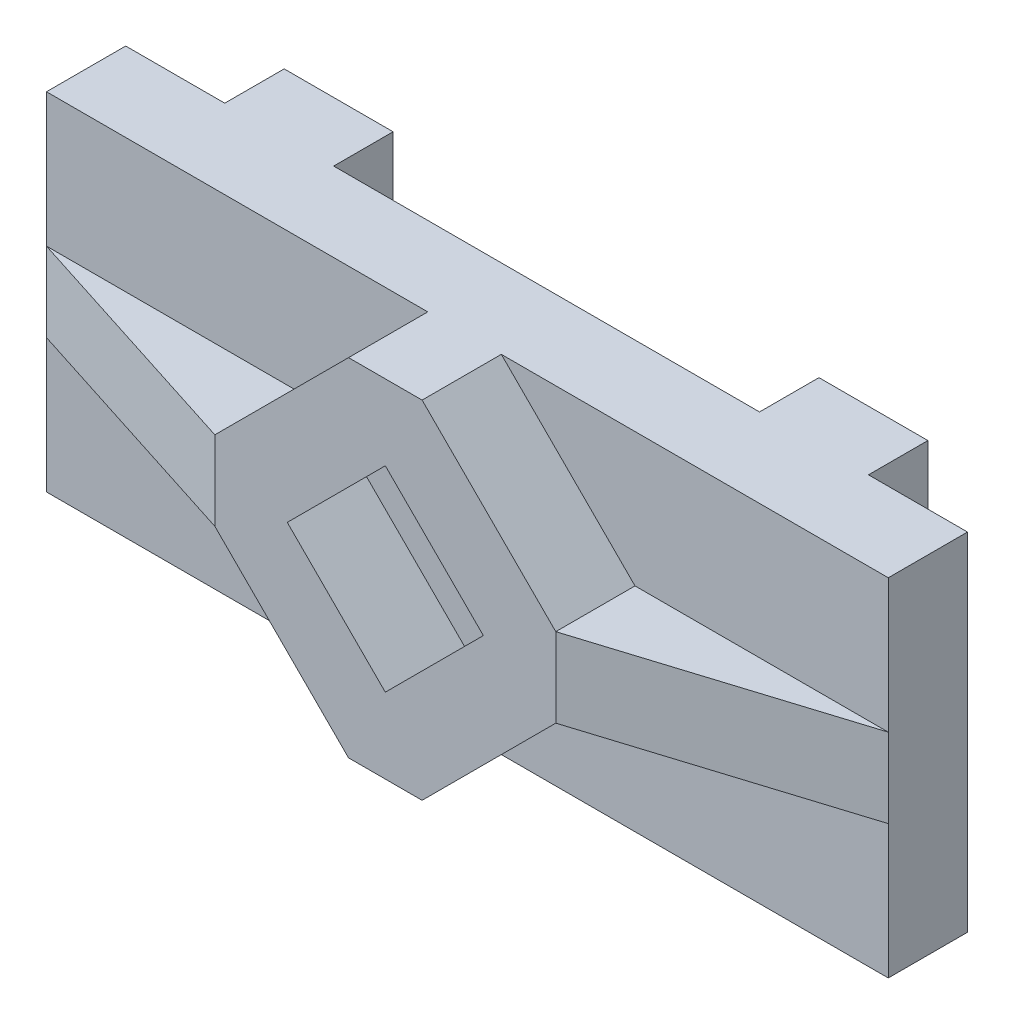
ISO-10303-21;
HEADER;
FILE_DESCRIPTION(('STEP AP214'),'2;1');
FILE_NAME('part.step','',(''),(''),'','','');
FILE_SCHEMA(('AUTOMOTIVE_DESIGN { 1 0 10303 214 1 1 1 1 }'));
ENDSEC;
DATA;
#1=APPLICATION_CONTEXT('core data for automotive mechanical design processes');
#2=APPLICATION_PROTOCOL_DEFINITION('international standard','automotive_design',2000,#1);
#3=PRODUCT_CONTEXT('',#1,'mechanical');
#4=PRODUCT('Part','Part','',(#3));
#5=PRODUCT_RELATED_PRODUCT_CATEGORY('part','',(#4));
#6=PRODUCT_DEFINITION_FORMATION('','',#4);
#7=PRODUCT_DEFINITION_CONTEXT('part definition',#1,'design');
#8=PRODUCT_DEFINITION('design','',#6,#7);
#9=PRODUCT_DEFINITION_SHAPE('','',#8);
#10=(LENGTH_UNIT() NAMED_UNIT(*) SI_UNIT(.MILLI.,.METRE.));
#11=(NAMED_UNIT(*) PLANE_ANGLE_UNIT() SI_UNIT($,.RADIAN.));
#12=(NAMED_UNIT(*) SI_UNIT($,.STERADIAN.) SOLID_ANGLE_UNIT());
#13=UNCERTAINTY_MEASURE_WITH_UNIT(LENGTH_MEASURE(1.E-05),#10,'distance_accuracy_value','');
#14=(GEOMETRIC_REPRESENTATION_CONTEXT(3) GLOBAL_UNCERTAINTY_ASSIGNED_CONTEXT((#13)) GLOBAL_UNIT_ASSIGNED_CONTEXT((#10,
#11,#12)) REPRESENTATION_CONTEXT('',''));
#15=CARTESIAN_POINT('',(0.,0.,0.));
#16=DIRECTION('',(0.,0.,1.));
#17=DIRECTION('',(1.,0.,0.));
#18=AXIS2_PLACEMENT_3D('',#15,#16,#17);
#19=CARTESIAN_POINT('',(0.,0.,0.));
#20=DIRECTION('',(0.,0.,1.));
#21=DIRECTION('',(1.,0.,0.));
#22=AXIS2_PLACEMENT_3D('',#19,#20,#21);
#23=PLANE('',#22);
#24=DIRECTION('',(1.,0.,0.));
#25=VECTOR('',#24,1.);
#26=CARTESIAN_POINT('',(0.,0.,0.));
#27=LINE('',#26,#25);
#28=CARTESIAN_POINT('',(150.,0.,0.));
#29=VERTEX_POINT('',#28);
#30=CARTESIAN_POINT('',(170.,0.,0.));
#31=VERTEX_POINT('',#30);
#32=EDGE_CURVE('E407',#29,#31,#27,.T.);
#33=ORIENTED_EDGE('',*,*,#32,.F.);
#34=DIRECTION('',(0.,-1.,0.));
#35=VECTOR('',#34,1.);
#36=CARTESIAN_POINT('',(150.,70.,0.));
#37=LINE('',#36,#35);
#38=CARTESIAN_POINT('',(150.,70.,0.));
#39=VERTEX_POINT('',#38);
#40=EDGE_CURVE('E247',#39,#29,#37,.T.);
#41=ORIENTED_EDGE('',*,*,#40,.F.);
#42=DIRECTION('',(-1.,0.,0.));
#43=VECTOR('',#42,1.);
#44=CARTESIAN_POINT('',(170.,70.,0.));
#45=LINE('',#44,#43);
#46=CARTESIAN_POINT('',(170.,70.,0.));
#47=VERTEX_POINT('',#46);
#48=EDGE_CURVE('E395',#47,#39,#45,.T.);
#49=ORIENTED_EDGE('',*,*,#48,.F.);
#50=DIRECTION('',(0.,1.,0.));
#51=VECTOR('',#50,1.);
#52=CARTESIAN_POINT('',(170.,0.,0.));
#53=LINE('',#52,#51);
#54=EDGE_CURVE('E408',#31,#47,#53,.T.);
#55=ORIENTED_EDGE('',*,*,#54,.F.);
#56=EDGE_LOOP('',(#33,#41,#49,#55));
#57=FACE_BOUND('',#56,.T.);
#58=ADVANCED_FACE('F50',(#57),#23,.F.);
#59=CARTESIAN_POINT('',(128.,70.,0.));
#60=VERTEX_POINT('',#59);
#61=CARTESIAN_POINT('',(42.,70.,0.));
#62=VERTEX_POINT('',#61);
#63=EDGE_CURVE('E414',#60,#62,#45,.T.);
#64=ORIENTED_EDGE('',*,*,#63,.F.);
#65=DIRECTION('',(0.,-1.,0.));
#66=VECTOR('',#65,1.);
#67=CARTESIAN_POINT('',(128.,70.,0.));
#68=LINE('',#67,#66);
#69=CARTESIAN_POINT('',(128.,0.,0.));
#70=VERTEX_POINT('',#69);
#71=EDGE_CURVE('E229',#60,#70,#68,.T.);
#72=ORIENTED_EDGE('',*,*,#71,.T.);
#73=CARTESIAN_POINT('',(42.,0.,0.));
#74=VERTEX_POINT('',#73);
#75=EDGE_CURVE('E411',#74,#70,#27,.T.);
#76=ORIENTED_EDGE('',*,*,#75,.F.);
#77=DIRECTION('',(0.,-1.,0.));
#78=VECTOR('',#77,1.);
#79=CARTESIAN_POINT('',(42.,70.,0.));
#80=LINE('',#79,#78);
#81=EDGE_CURVE('E267',#62,#74,#80,.T.);
#82=ORIENTED_EDGE('',*,*,#81,.F.);
#83=EDGE_LOOP('',(#64,#72,#76,#82));
#84=FACE_BOUND('',#83,.T.);
#85=ADVANCED_FACE('F500',(#84),#23,.F.);
#86=CARTESIAN_POINT('',(0.,0.,16.));
#87=DIRECTION('',(0.,0.,1.));
#88=DIRECTION('',(1.,0.,0.));
#89=AXIS2_PLACEMENT_3D('',#86,#87,#88);
#90=PLANE('',#89);
#91=DIRECTION('',(0.707106781186548,-0.707106781186548,0.));
#92=VECTOR('',#91,1.);
#93=CARTESIAN_POINT('',(38.5,38.5,16.));
#94=LINE('',#93,#92);
#95=CARTESIAN_POINT('',(50.,27.,16.));
#96=VERTEX_POINT('',#95);
#97=CARTESIAN_POINT('',(77.,0.,16.));
#98=VERTEX_POINT('',#97);
#99=EDGE_CURVE('E338',#96,#98,#94,.T.);
#100=ORIENTED_EDGE('',*,*,#99,.F.);
#101=DIRECTION('',(1.,0.,0.));
#102=VECTOR('',#101,1.);
#103=CARTESIAN_POINT('',(50.,27.,16.));
#104=LINE('',#103,#102);
#105=CARTESIAN_POINT('',(0.,27.,16.));
#106=VERTEX_POINT('',#105);
#107=EDGE_CURVE('E276',#106,#96,#104,.T.);
#108=ORIENTED_EDGE('',*,*,#107,.F.);
#109=DIRECTION('',(0.,-1.,0.));
#110=VECTOR('',#109,1.);
#111=CARTESIAN_POINT('',(0.,27.,16.));
#112=LINE('',#111,#110);
#113=CARTESIAN_POINT('',(0.,0.,16.));
#114=VERTEX_POINT('',#113);
#115=EDGE_CURVE('E281',#106,#114,#112,.T.);
#116=ORIENTED_EDGE('',*,*,#115,.T.);
#117=DIRECTION('',(1.,0.,0.));
#118=VECTOR('',#117,1.);
#119=CARTESIAN_POINT('',(0.,0.,16.));
#120=LINE('',#119,#118);
#121=EDGE_CURVE('E392',#114,#98,#120,.T.);
#122=ORIENTED_EDGE('',*,*,#121,.T.);
#123=EDGE_LOOP('',(#100,#108,#116,#122));
#124=FACE_BOUND('',#123,.T.);
#125=ADVANCED_FACE('F471',(#124),#90,.T.);
#126=CARTESIAN_POINT('',(170.,43.,16.));
#127=DIRECTION('',(0.298555546721857,0.,0.954392259776667));
#128=DIRECTION('',(0.954392259776667,0.,-0.298555546721857));
#129=AXIS2_PLACEMENT_3D('',#126,#127,#128);
#130=PLANE('',#129);
#131=DIRECTION('',(0.,-1.,0.));
#132=VECTOR('',#131,1.);
#133=CARTESIAN_POINT('',(118.852813742386,-1.03088383092408E-13,32.));
#134=LINE('',#133,#132);
#135=CARTESIAN_POINT('',(118.852813742386,43.,32.));
#136=VERTEX_POINT('',#135);
#137=CARTESIAN_POINT('',(118.852813742386,27.,32.));
#138=VERTEX_POINT('',#137);
#139=EDGE_CURVE('E339',#136,#138,#134,.T.);
#140=ORIENTED_EDGE('',*,*,#139,.T.);
#141=DIRECTION('',(-0.954392259776667,0.,0.298555546721857));
#142=VECTOR('',#141,1.);
#143=CARTESIAN_POINT('',(170.,27.,16.));
#144=LINE('',#143,#142);
#145=CARTESIAN_POINT('',(170.,27.,16.));
#146=VERTEX_POINT('',#145);
#147=EDGE_CURVE('E292',#146,#138,#144,.T.);
#148=ORIENTED_EDGE('',*,*,#147,.F.);
#149=DIRECTION('',(0.,1.,0.));
#150=VECTOR('',#149,1.);
#151=CARTESIAN_POINT('',(170.,0.,16.));
#152=LINE('',#151,#150);
#153=CARTESIAN_POINT('',(170.,43.,16.));
#154=VERTEX_POINT('',#153);
#155=EDGE_CURVE('E397',#146,#154,#152,.T.);
#156=ORIENTED_EDGE('',*,*,#155,.T.);
#157=DIRECTION('',(-0.954392259776667,0.,0.298555546721857));
#158=VECTOR('',#157,1.);
#159=CARTESIAN_POINT('',(170.,43.,16.));
#160=LINE('',#159,#158);
#161=EDGE_CURVE('E300',#154,#136,#160,.T.);
#162=ORIENTED_EDGE('',*,*,#161,.T.);
#163=EDGE_LOOP('',(#140,#148,#156,#162));
#164=FACE_BOUND('',#163,.T.);
#165=ADVANCED_FACE('F442',(#164),#130,.T.);
#166=DIRECTION('',(0.707106781186547,-0.707106781186548,0.));
#167=VECTOR('',#166,1.);
#168=CARTESIAN_POINT('',(80.9264068711929,80.9264068711928,16.));
#169=LINE('',#168,#167);
#170=CARTESIAN_POINT('',(91.8528137423857,70.,16.));
#171=VERTEX_POINT('',#170);
#172=CARTESIAN_POINT('',(118.852813742386,43.,16.));
#173=VERTEX_POINT('',#172);
#174=EDGE_CURVE('E363',#171,#173,#169,.T.);
#175=ORIENTED_EDGE('',*,*,#174,.T.);
#176=DIRECTION('',(1.,0.,0.));
#177=VECTOR('',#176,1.);
#178=CARTESIAN_POINT('',(118.852813742386,43.,16.));
#179=LINE('',#178,#177);
#180=EDGE_CURVE('E297',#173,#154,#179,.T.);
#181=ORIENTED_EDGE('',*,*,#180,.T.);
#182=CARTESIAN_POINT('',(170.,70.,16.));
#183=VERTEX_POINT('',#182);
#184=EDGE_CURVE('E394',#154,#183,#152,.T.);
#185=ORIENTED_EDGE('',*,*,#184,.T.);
#186=DIRECTION('',(-1.,0.,0.));
#187=VECTOR('',#186,1.);
#188=CARTESIAN_POINT('',(170.,70.,16.));
#189=LINE('',#188,#187);
#190=EDGE_CURVE('E399',#183,#171,#189,.T.);
#191=ORIENTED_EDGE('',*,*,#190,.T.);
#192=EDGE_LOOP('',(#175,#181,#185,#191));
#193=FACE_BOUND('',#192,.T.);
#194=ADVANCED_FACE('F444',(#193),#90,.T.);
#195=CARTESIAN_POINT('',(91.8528137423857,0.,16.));
#196=VERTEX_POINT('',#195);
#197=CARTESIAN_POINT('',(170.,0.,16.));
#198=VERTEX_POINT('',#197);
#199=EDGE_CURVE('E391',#196,#198,#120,.T.);
#200=ORIENTED_EDGE('',*,*,#199,.T.);
#201=EDGE_CURVE('E398',#198,#146,#152,.T.);
#202=ORIENTED_EDGE('',*,*,#201,.T.);
#203=DIRECTION('',(1.,0.,0.));
#204=VECTOR('',#203,1.);
#205=CARTESIAN_POINT('',(118.852813742386,27.,16.));
#206=LINE('',#205,#204);
#207=CARTESIAN_POINT('',(118.852813742386,27.,16.));
#208=VERTEX_POINT('',#207);
#209=EDGE_CURVE('E295',#208,#146,#206,.T.);
#210=ORIENTED_EDGE('',*,*,#209,.F.);
#211=DIRECTION('',(-0.707106781186548,-0.707106781186548,0.));
#212=VECTOR('',#211,1.);
#213=CARTESIAN_POINT('',(45.9264068711928,-45.9264068711928,16.));
#214=LINE('',#213,#212);
#215=EDGE_CURVE('E328',#208,#196,#214,.T.);
#216=ORIENTED_EDGE('',*,*,#215,.T.);
#217=EDGE_LOOP('',(#200,#202,#210,#216));
#218=FACE_BOUND('',#217,.T.);
#219=ADVANCED_FACE('F464',(#218),#90,.T.);
#220=CARTESIAN_POINT('',(0.,70.,16.));
#221=DIRECTION('',(1.,0.,0.));
#222=DIRECTION('',(0.,0.,-1.));
#223=AXIS2_PLACEMENT_3D('',#220,#221,#222);
#224=PLANE('',#223);
#225=DIRECTION('',(0.,-1.,0.));
#226=VECTOR('',#225,1.);
#227=CARTESIAN_POINT('',(0.,70.,0.));
#228=LINE('',#227,#226);
#229=CARTESIAN_POINT('',(0.,70.,0.));
#230=VERTEX_POINT('',#229);
#231=CARTESIAN_POINT('',(0.,0.,0.));
#232=VERTEX_POINT('',#231);
#233=EDGE_CURVE('E390',#230,#232,#228,.T.);
#234=ORIENTED_EDGE('',*,*,#233,.T.);
#235=DIRECTION('',(0.,0.,-1.));
#236=VECTOR('',#235,1.);
#237=CARTESIAN_POINT('',(0.,0.,16.));
#238=LINE('',#237,#236);
#239=EDGE_CURVE('E11',#114,#232,#238,.T.);
#240=ORIENTED_EDGE('',*,*,#239,.F.);
#241=ORIENTED_EDGE('',*,*,#115,.F.);
#242=DIRECTION('',(0.,-1.,0.));
#243=VECTOR('',#242,1.);
#244=CARTESIAN_POINT('',(0.,43.,16.));
#245=LINE('',#244,#243);
#246=CARTESIAN_POINT('',(0.,43.,16.));
#247=VERTEX_POINT('',#246);
#248=EDGE_CURVE('E287',#247,#106,#245,.T.);
#249=ORIENTED_EDGE('',*,*,#248,.F.);
#250=DIRECTION('',(0.,-1.,0.));
#251=VECTOR('',#250,1.);
#252=CARTESIAN_POINT('',(0.,70.,16.));
#253=LINE('',#252,#251);
#254=CARTESIAN_POINT('',(0.,70.,16.));
#255=VERTEX_POINT('',#254);
#256=EDGE_CURVE('E389',#255,#247,#253,.T.);
#257=ORIENTED_EDGE('',*,*,#256,.F.);
#258=DIRECTION('',(0.,0.,-1.));
#259=VECTOR('',#258,1.);
#260=CARTESIAN_POINT('',(0.,70.,16.));
#261=LINE('',#260,#259);
#262=EDGE_CURVE('E401',#255,#230,#261,.T.);
#263=ORIENTED_EDGE('',*,*,#262,.T.);
#264=EDGE_LOOP('',(#234,#240,#241,#249,#257,#263));
#265=FACE_BOUND('',#264,.T.);
#266=ADVANCED_FACE('F47',(#265),#224,.F.);
#267=CARTESIAN_POINT('',(0.,0.,16.));
#268=DIRECTION('',(0.,1.,0.));
#269=DIRECTION('',(0.,0.,1.));
#270=AXIS2_PLACEMENT_3D('',#267,#268,#269);
#271=PLANE('',#270);
#272=ORIENTED_EDGE('',*,*,#121,.F.);
#273=ORIENTED_EDGE('',*,*,#239,.T.);
#274=CARTESIAN_POINT('',(20.,0.,0.));
#275=VERTEX_POINT('',#274);
#276=EDGE_CURVE('E410',#232,#275,#27,.T.);
#277=ORIENTED_EDGE('',*,*,#276,.T.);
#278=DIRECTION('',(0.,0.,-1.));
#279=VECTOR('',#278,1.);
#280=CARTESIAN_POINT('',(20.,0.,0.));
#281=LINE('',#280,#279);
#282=CARTESIAN_POINT('',(20.,0.,-12.));
#283=VERTEX_POINT('',#282);
#284=EDGE_CURVE('E69',#275,#283,#281,.T.);
#285=ORIENTED_EDGE('',*,*,#284,.T.);
#286=DIRECTION('',(1.,0.,0.));
#287=VECTOR('',#286,1.);
#288=CARTESIAN_POINT('',(20.,0.,-12.));
#289=LINE('',#288,#287);
#290=CARTESIAN_POINT('',(42.,0.,-12.));
#291=VERTEX_POINT('',#290);
#292=EDGE_CURVE('E263',#283,#291,#289,.T.);
#293=ORIENTED_EDGE('',*,*,#292,.T.);
#294=DIRECTION('',(0.,0.,1.));
#295=VECTOR('',#294,1.);
#296=CARTESIAN_POINT('',(42.,0.,-12.));
#297=LINE('',#296,#295);
#298=EDGE_CURVE('E257',#291,#74,#297,.T.);
#299=ORIENTED_EDGE('',*,*,#298,.T.);
#300=ORIENTED_EDGE('',*,*,#75,.T.);
#301=DIRECTION('',(0.,0.,-1.));
#302=VECTOR('',#301,1.);
#303=CARTESIAN_POINT('',(128.,0.,-12.));
#304=LINE('',#303,#302);
#305=CARTESIAN_POINT('',(128.,0.,-12.));
#306=VERTEX_POINT('',#305);
#307=EDGE_CURVE('E244',#70,#306,#304,.T.);
#308=ORIENTED_EDGE('',*,*,#307,.T.);
#309=DIRECTION('',(1.,0.,0.));
#310=VECTOR('',#309,1.);
#311=CARTESIAN_POINT('',(150.,0.,-12.));
#312=LINE('',#311,#310);
#313=CARTESIAN_POINT('',(150.,0.,-12.));
#314=VERTEX_POINT('',#313);
#315=EDGE_CURVE('E228',#306,#314,#312,.T.);
#316=ORIENTED_EDGE('',*,*,#315,.T.);
#317=DIRECTION('',(0.,0.,1.));
#318=VECTOR('',#317,1.);
#319=CARTESIAN_POINT('',(150.,0.,0.));
#320=LINE('',#319,#318);
#321=EDGE_CURVE('E237',#314,#29,#320,.T.);
#322=ORIENTED_EDGE('',*,*,#321,.T.);
#323=ORIENTED_EDGE('',*,*,#32,.T.);
#324=DIRECTION('',(0.,0.,-1.));
#325=VECTOR('',#324,1.);
#326=CARTESIAN_POINT('',(170.,0.,16.));
#327=LINE('',#326,#325);
#328=EDGE_CURVE('E54',#198,#31,#327,.T.);
#329=ORIENTED_EDGE('',*,*,#328,.F.);
#330=ORIENTED_EDGE('',*,*,#199,.F.);
#331=DIRECTION('',(0.,0.,-1.));
#332=VECTOR('',#331,1.);
#333=CARTESIAN_POINT('',(91.8528137423857,0.,32.));
#334=LINE('',#333,#332);
#335=CARTESIAN_POINT('',(91.8528137423857,0.,32.));
#336=VERTEX_POINT('',#335);
#337=EDGE_CURVE('E356',#336,#196,#334,.T.);
#338=ORIENTED_EDGE('',*,*,#337,.F.);
#339=DIRECTION('',(1.,0.,0.));
#340=VECTOR('',#339,1.);
#341=CARTESIAN_POINT('',(0.,0.,32.));
#342=LINE('',#341,#340);
#343=CARTESIAN_POINT('',(77.,0.,32.));
#344=VERTEX_POINT('',#343);
#345=EDGE_CURVE('E358',#344,#336,#342,.T.);
#346=ORIENTED_EDGE('',*,*,#345,.F.);
#347=DIRECTION('',(0.,0.,-1.));
#348=VECTOR('',#347,1.);
#349=CARTESIAN_POINT('',(77.,0.,32.));
#350=LINE('',#349,#348);
#351=EDGE_CURVE('E369',#344,#98,#350,.T.);
#352=ORIENTED_EDGE('',*,*,#351,.T.);
#353=EDGE_LOOP('',(#272,#273,#277,#285,#293,#299,#300,#308,#316,#322,#323,#329,#330,#338,#346,#352));
#354=FACE_BOUND('',#353,.T.);
#355=ADVANCED_FACE('F467',(#354),#271,.F.);
#356=CARTESIAN_POINT('',(170.,0.,16.));
#357=DIRECTION('',(-1.,0.,0.));
#358=DIRECTION('',(0.,0.,1.));
#359=AXIS2_PLACEMENT_3D('',#356,#357,#358);
#360=PLANE('',#359);
#361=ORIENTED_EDGE('',*,*,#54,.T.);
#362=DIRECTION('',(0.,0.,-1.));
#363=VECTOR('',#362,1.);
#364=CARTESIAN_POINT('',(170.,70.,16.));
#365=LINE('',#364,#363);
#366=EDGE_CURVE('E416',#183,#47,#365,.T.);
#367=ORIENTED_EDGE('',*,*,#366,.F.);
#368=ORIENTED_EDGE('',*,*,#184,.F.);
#369=ORIENTED_EDGE('',*,*,#155,.F.);
#370=ORIENTED_EDGE('',*,*,#201,.F.);
#371=ORIENTED_EDGE('',*,*,#328,.T.);
#372=EDGE_LOOP('',(#361,#367,#368,#369,#370,#371));
#373=FACE_BOUND('',#372,.T.);
#374=ADVANCED_FACE('F424',(#373),#360,.F.);
#375=CARTESIAN_POINT('',(170.,70.,16.));
#376=DIRECTION('',(0.,-1.,0.));
#377=DIRECTION('',(0.,0.,-1.));
#378=AXIS2_PLACEMENT_3D('',#375,#376,#377);
#379=PLANE('',#378);
#380=ORIENTED_EDGE('',*,*,#48,.T.);
#381=DIRECTION('',(0.,0.,1.));
#382=VECTOR('',#381,1.);
#383=CARTESIAN_POINT('',(150.,70.,0.));
#384=LINE('',#383,#382);
#385=CARTESIAN_POINT('',(150.,70.,-12.));
#386=VERTEX_POINT('',#385);
#387=EDGE_CURVE('E234',#386,#39,#384,.T.);
#388=ORIENTED_EDGE('',*,*,#387,.F.);
#389=DIRECTION('',(1.,0.,0.));
#390=VECTOR('',#389,1.);
#391=CARTESIAN_POINT('',(150.,70.,-12.));
#392=LINE('',#391,#390);
#393=CARTESIAN_POINT('',(128.,70.,-12.));
#394=VERTEX_POINT('',#393);
#395=EDGE_CURVE('E221',#394,#386,#392,.T.);
#396=ORIENTED_EDGE('',*,*,#395,.F.);
#397=DIRECTION('',(0.,0.,-1.));
#398=VECTOR('',#397,1.);
#399=CARTESIAN_POINT('',(128.,70.,-12.));
#400=LINE('',#399,#398);
#401=EDGE_CURVE('E65',#60,#394,#400,.T.);
#402=ORIENTED_EDGE('',*,*,#401,.F.);
#403=ORIENTED_EDGE('',*,*,#63,.T.);
#404=DIRECTION('',(0.,0.,1.));
#405=VECTOR('',#404,1.);
#406=CARTESIAN_POINT('',(42.,70.,-12.));
#407=LINE('',#406,#405);
#408=CARTESIAN_POINT('',(42.,70.,-12.));
#409=VERTEX_POINT('',#408);
#410=EDGE_CURVE('E256',#409,#62,#407,.T.);
#411=ORIENTED_EDGE('',*,*,#410,.F.);
#412=DIRECTION('',(1.,0.,0.));
#413=VECTOR('',#412,1.);
#414=CARTESIAN_POINT('',(20.,70.,-12.));
#415=LINE('',#414,#413);
#416=CARTESIAN_POINT('',(20.,70.,-12.));
#417=VERTEX_POINT('',#416);
#418=EDGE_CURVE('E253',#417,#409,#415,.T.);
#419=ORIENTED_EDGE('',*,*,#418,.F.);
#420=DIRECTION('',(0.,0.,-1.));
#421=VECTOR('',#420,1.);
#422=CARTESIAN_POINT('',(20.,70.,0.));
#423=LINE('',#422,#421);
#424=CARTESIAN_POINT('',(20.,70.,0.));
#425=VERTEX_POINT('',#424);
#426=EDGE_CURVE('E255',#425,#417,#423,.T.);
#427=ORIENTED_EDGE('',*,*,#426,.F.);
#428=EDGE_CURVE('E412',#425,#230,#45,.T.);
#429=ORIENTED_EDGE('',*,*,#428,.T.);
#430=ORIENTED_EDGE('',*,*,#262,.F.);
#431=CARTESIAN_POINT('',(77.,70.,16.));
#432=VERTEX_POINT('',#431);
#433=EDGE_CURVE('E396',#432,#255,#189,.T.);
#434=ORIENTED_EDGE('',*,*,#433,.F.);
#435=DIRECTION('',(0.,0.,-1.));
#436=VECTOR('',#435,1.);
#437=CARTESIAN_POINT('',(77.,70.,32.));
#438=LINE('',#437,#436);
#439=CARTESIAN_POINT('',(77.,70.,32.));
#440=VERTEX_POINT('',#439);
#441=EDGE_CURVE('E378',#440,#432,#438,.T.);
#442=ORIENTED_EDGE('',*,*,#441,.F.);
#443=DIRECTION('',(-1.,0.,0.));
#444=VECTOR('',#443,1.);
#445=CARTESIAN_POINT('',(0.,70.,32.));
#446=LINE('',#445,#444);
#447=CARTESIAN_POINT('',(91.8528137423857,70.,32.));
#448=VERTEX_POINT('',#447);
#449=EDGE_CURVE('E346',#448,#440,#446,.T.);
#450=ORIENTED_EDGE('',*,*,#449,.F.);
#451=DIRECTION('',(0.,0.,-1.));
#452=VECTOR('',#451,1.);
#453=CARTESIAN_POINT('',(91.8528137423857,70.,32.));
#454=LINE('',#453,#452);
#455=EDGE_CURVE('E382',#448,#171,#454,.T.);
#456=ORIENTED_EDGE('',*,*,#455,.T.);
#457=ORIENTED_EDGE('',*,*,#190,.F.);
#458=ORIENTED_EDGE('',*,*,#366,.T.);
#459=EDGE_LOOP('',(#380,#388,#396,#402,#403,#411,#419,#427,#429,#430,#434,#442,#450,#456,#457,#458));
#460=FACE_BOUND('',#459,.T.);
#461=ADVANCED_FACE('F231',(#460),#379,.F.);
#462=DIRECTION('',(1.,0.,0.));
#463=VECTOR('',#462,1.);
#464=CARTESIAN_POINT('',(50.,43.,16.));
#465=LINE('',#464,#463);
#466=CARTESIAN_POINT('',(50.,43.,16.));
#467=VERTEX_POINT('',#466);
#468=EDGE_CURVE('E290',#247,#467,#465,.T.);
#469=ORIENTED_EDGE('',*,*,#468,.T.);
#470=DIRECTION('',(-0.707106781186548,-0.707106781186548,0.));
#471=VECTOR('',#470,1.);
#472=CARTESIAN_POINT('',(3.50000000000001,-3.50000000000001,16.));
#473=LINE('',#472,#471);
#474=EDGE_CURVE('E364',#432,#467,#473,.T.);
#475=ORIENTED_EDGE('',*,*,#474,.F.);
#476=ORIENTED_EDGE('',*,*,#433,.T.);
#477=ORIENTED_EDGE('',*,*,#256,.T.);
#478=EDGE_LOOP('',(#469,#475,#476,#477));
#479=FACE_BOUND('',#478,.T.);
#480=ADVANCED_FACE('F519',(#479),#90,.T.);
#481=ORIENTED_EDGE('',*,*,#428,.F.);
#482=DIRECTION('',(0.,-1.,0.));
#483=VECTOR('',#482,1.);
#484=CARTESIAN_POINT('',(20.,70.,0.));
#485=LINE('',#484,#483);
#486=EDGE_CURVE('E265',#425,#275,#485,.T.);
#487=ORIENTED_EDGE('',*,*,#486,.T.);
#488=ORIENTED_EDGE('',*,*,#276,.F.);
#489=ORIENTED_EDGE('',*,*,#233,.F.);
#490=EDGE_LOOP('',(#481,#487,#488,#489));
#491=FACE_BOUND('',#490,.T.);
#492=ADVANCED_FACE('F483',(#491),#23,.F.);
#493=CARTESIAN_POINT('',(45.9264068711928,-45.9264068711928,32.));
#494=DIRECTION('',(0.707106781186547,-0.707106781186547,0.));
#495=DIRECTION('',(0.707106781186548,0.707106781186548,0.));
#496=AXIS2_PLACEMENT_3D('',#493,#494,#495);
#497=PLANE('',#496);
#498=ORIENTED_EDGE('',*,*,#215,.F.);
#499=DIRECTION('',(0.,0.,-1.));
#500=VECTOR('',#499,1.);
#501=CARTESIAN_POINT('',(118.852813742386,27.,32.));
#502=LINE('',#501,#500);
#503=EDGE_CURVE('E383',#138,#208,#502,.T.);
#504=ORIENTED_EDGE('',*,*,#503,.F.);
#505=DIRECTION('',(-0.707106781186548,-0.707106781186548,0.));
#506=VECTOR('',#505,1.);
#507=CARTESIAN_POINT('',(45.9264068711928,-45.9264068711928,32.));
#508=LINE('',#507,#506);
#509=EDGE_CURVE('E337',#138,#336,#508,.T.);
#510=ORIENTED_EDGE('',*,*,#509,.T.);
#511=ORIENTED_EDGE('',*,*,#337,.T.);
#512=EDGE_LOOP('',(#498,#504,#510,#511));
#513=FACE_BOUND('',#512,.T.);
#514=ADVANCED_FACE('F459',(#513),#497,.T.);
#515=CARTESIAN_POINT('',(80.9264068711929,80.9264068711928,32.));
#516=DIRECTION('',(0.707106781186548,0.707106781186547,0.));
#517=DIRECTION('',(-0.707106781186547,0.707106781186548,0.));
#518=AXIS2_PLACEMENT_3D('',#515,#516,#517);
#519=PLANE('',#518);
#520=ORIENTED_EDGE('',*,*,#174,.F.);
#521=ORIENTED_EDGE('',*,*,#455,.F.);
#522=DIRECTION('',(0.707106781186547,-0.707106781186548,0.));
#523=VECTOR('',#522,1.);
#524=CARTESIAN_POINT('',(80.9264068711929,80.9264068711928,32.));
#525=LINE('',#524,#523);
#526=EDGE_CURVE('E344',#448,#136,#525,.T.);
#527=ORIENTED_EDGE('',*,*,#526,.T.);
#528=DIRECTION('',(0.,0.,-1.));
#529=VECTOR('',#528,1.);
#530=CARTESIAN_POINT('',(118.852813742386,43.,32.));
#531=LINE('',#530,#529);
#532=EDGE_CURVE('E384',#136,#173,#531,.T.);
#533=ORIENTED_EDGE('',*,*,#532,.T.);
#534=EDGE_LOOP('',(#520,#521,#527,#533));
#535=FACE_BOUND('',#534,.T.);
#536=ADVANCED_FACE('F449',(#535),#519,.T.);
#537=CARTESIAN_POINT('',(3.50000000000001,-3.50000000000001,32.));
#538=DIRECTION('',(0.707106781186547,-0.707106781186547,0.));
#539=DIRECTION('',(0.707106781186548,0.707106781186548,0.));
#540=AXIS2_PLACEMENT_3D('',#537,#538,#539);
#541=PLANE('',#540);
#542=ORIENTED_EDGE('',*,*,#474,.T.);
#543=DIRECTION('',(0.,0.,-1.));
#544=VECTOR('',#543,1.);
#545=CARTESIAN_POINT('',(50.,43.,32.));
#546=LINE('',#545,#544);
#547=CARTESIAN_POINT('',(50.,43.,32.));
#548=VERTEX_POINT('',#547);
#549=EDGE_CURVE('E376',#548,#467,#546,.T.);
#550=ORIENTED_EDGE('',*,*,#549,.F.);
#551=DIRECTION('',(-0.707106781186548,-0.707106781186548,0.));
#552=VECTOR('',#551,1.);
#553=CARTESIAN_POINT('',(3.50000000000001,-3.50000000000001,32.));
#554=LINE('',#553,#552);
#555=EDGE_CURVE('E347',#440,#548,#554,.T.);
#556=ORIENTED_EDGE('',*,*,#555,.F.);
#557=ORIENTED_EDGE('',*,*,#441,.T.);
#558=EDGE_LOOP('',(#542,#550,#556,#557));
#559=FACE_BOUND('',#558,.T.);
#560=ADVANCED_FACE('F574',(#559),#541,.F.);
#561=CARTESIAN_POINT('',(38.5,38.5,32.));
#562=DIRECTION('',(0.707106781186547,0.707106781186547,0.));
#563=DIRECTION('',(-0.707106781186548,0.707106781186548,0.));
#564=AXIS2_PLACEMENT_3D('',#561,#562,#563);
#565=PLANE('',#564);
#566=ORIENTED_EDGE('',*,*,#99,.T.);
#567=ORIENTED_EDGE('',*,*,#351,.F.);
#568=DIRECTION('',(0.707106781186548,-0.707106781186548,0.));
#569=VECTOR('',#568,1.);
#570=CARTESIAN_POINT('',(38.5,38.5,32.));
#571=LINE('',#570,#569);
#572=CARTESIAN_POINT('',(50.,27.,32.));
#573=VERTEX_POINT('',#572);
#574=EDGE_CURVE('E352',#573,#344,#571,.T.);
#575=ORIENTED_EDGE('',*,*,#574,.F.);
#576=DIRECTION('',(0.,0.,-1.));
#577=VECTOR('',#576,1.);
#578=CARTESIAN_POINT('',(50.,27.,32.));
#579=LINE('',#578,#577);
#580=EDGE_CURVE('E373',#573,#96,#579,.T.);
#581=ORIENTED_EDGE('',*,*,#580,.T.);
#582=EDGE_LOOP('',(#566,#567,#575,#581));
#583=FACE_BOUND('',#582,.T.);
#584=ADVANCED_FACE('F468',(#583),#565,.F.);
#585=CARTESIAN_POINT('',(0.,0.,32.));
#586=DIRECTION('',(0.,0.,1.));
#587=DIRECTION('',(1.,0.,0.));
#588=AXIS2_PLACEMENT_3D('',#585,#586,#587);
#589=PLANE('',#588);
#590=DIRECTION('',(-0.707106781186548,0.707106781186547,0.));
#591=VECTOR('',#590,1.);
#592=CARTESIAN_POINT('',(104.225396744416,35.,32.));
#593=LINE('',#592,#591);
#594=CARTESIAN_POINT('',(104.225396744416,35.,32.));
#595=VERTEX_POINT('',#594);
#596=CARTESIAN_POINT('',(84.4264068711929,54.7989898732233,32.));
#597=VERTEX_POINT('',#596);
#598=EDGE_CURVE('E303',#595,#597,#593,.T.);
#599=ORIENTED_EDGE('',*,*,#598,.F.);
#600=DIRECTION('',(0.707106781186547,0.707106781186548,0.));
#601=VECTOR('',#600,1.);
#602=CARTESIAN_POINT('',(84.4264068711929,15.2010101267767,32.));
#603=LINE('',#602,#601);
#604=CARTESIAN_POINT('',(84.4264068711929,15.2010101267767,32.));
#605=VERTEX_POINT('',#604);
#606=EDGE_CURVE('E308',#605,#595,#603,.T.);
#607=ORIENTED_EDGE('',*,*,#606,.F.);
#608=DIRECTION('',(0.707106781186548,-0.707106781186547,0.));
#609=VECTOR('',#608,1.);
#610=CARTESIAN_POINT('',(84.4264068711929,15.2010101267767,32.));
#611=LINE('',#610,#609);
#612=CARTESIAN_POINT('',(64.6274169979695,35.,32.));
#613=VERTEX_POINT('',#612);
#614=EDGE_CURVE('E325',#613,#605,#611,.T.);
#615=ORIENTED_EDGE('',*,*,#614,.F.);
#616=DIRECTION('',(-0.707106781186548,-0.707106781186547,0.));
#617=VECTOR('',#616,1.);
#618=CARTESIAN_POINT('',(84.4264068711929,54.7989898732233,32.));
#619=LINE('',#618,#617);
#620=EDGE_CURVE('E316',#597,#613,#619,.T.);
#621=ORIENTED_EDGE('',*,*,#620,.F.);
#622=EDGE_LOOP('',(#599,#607,#615,#621));
#623=FACE_BOUND('',#622,.T.);
#624=ORIENTED_EDGE('',*,*,#509,.F.);
#625=ORIENTED_EDGE('',*,*,#139,.F.);
#626=ORIENTED_EDGE('',*,*,#526,.F.);
#627=ORIENTED_EDGE('',*,*,#449,.T.);
#628=ORIENTED_EDGE('',*,*,#555,.T.);
#629=DIRECTION('',(0.,1.,0.));
#630=VECTOR('',#629,1.);
#631=CARTESIAN_POINT('',(50.,0.,32.));
#632=LINE('',#631,#630);
#633=EDGE_CURVE('E353',#573,#548,#632,.T.);
#634=ORIENTED_EDGE('',*,*,#633,.F.);
#635=ORIENTED_EDGE('',*,*,#574,.T.);
#636=ORIENTED_EDGE('',*,*,#345,.T.);
#637=EDGE_LOOP('',(#624,#625,#626,#627,#628,#634,#635,#636));
#638=FACE_BOUND('',#637,.T.);
#639=ADVANCED_FACE('F454',(#623,#638),#589,.T.);
#640=CARTESIAN_POINT('',(104.225396744416,35.,16.));
#641=DIRECTION('',(0.707106781186547,0.707106781186548,0.));
#642=DIRECTION('',(-0.707106781186548,0.707106781186547,0.));
#643=AXIS2_PLACEMENT_3D('',#640,#641,#642);
#644=PLANE('',#643);
#645=ORIENTED_EDGE('',*,*,#598,.T.);
#646=DIRECTION('',(0.,0.,1.));
#647=VECTOR('',#646,1.);
#648=CARTESIAN_POINT('',(84.4264068711929,54.7989898732233,16.));
#649=LINE('',#648,#647);
#650=CARTESIAN_POINT('',(84.4264068711929,54.7989898732233,16.));
#651=VERTEX_POINT('',#650);
#652=EDGE_CURVE('E320',#651,#597,#649,.T.);
#653=ORIENTED_EDGE('',*,*,#652,.F.);
#654=DIRECTION('',(-0.707106781186548,0.707106781186547,0.));
#655=VECTOR('',#654,1.);
#656=CARTESIAN_POINT('',(104.225396744416,35.,16.));
#657=LINE('',#656,#655);
#658=CARTESIAN_POINT('',(104.225396744416,35.,16.));
#659=VERTEX_POINT('',#658);
#660=EDGE_CURVE('E302',#659,#651,#657,.T.);
#661=ORIENTED_EDGE('',*,*,#660,.F.);
#662=DIRECTION('',(0.,0.,1.));
#663=VECTOR('',#662,1.);
#664=CARTESIAN_POINT('',(104.225396744416,35.,16.));
#665=LINE('',#664,#663);
#666=EDGE_CURVE('E330',#659,#595,#665,.T.);
#667=ORIENTED_EDGE('',*,*,#666,.T.);
#668=EDGE_LOOP('',(#645,#653,#661,#667));
#669=FACE_BOUND('',#668,.T.);
#670=ADVANCED_FACE('F557',(#669),#644,.F.);
#671=CARTESIAN_POINT('',(84.4264068711929,15.2010101267767,16.));
#672=DIRECTION('',(0.707106781186548,-0.707106781186547,0.));
#673=DIRECTION('',(0.707106781186547,0.707106781186548,0.));
#674=AXIS2_PLACEMENT_3D('',#671,#672,#673);
#675=PLANE('',#674);
#676=ORIENTED_EDGE('',*,*,#606,.T.);
#677=ORIENTED_EDGE('',*,*,#666,.F.);
#678=DIRECTION('',(0.707106781186547,0.707106781186548,0.));
#679=VECTOR('',#678,1.);
#680=CARTESIAN_POINT('',(84.4264068711929,15.2010101267767,16.));
#681=LINE('',#680,#679);
#682=CARTESIAN_POINT('',(84.4264068711929,15.2010101267767,16.));
#683=VERTEX_POINT('',#682);
#684=EDGE_CURVE('E313',#683,#659,#681,.T.);
#685=ORIENTED_EDGE('',*,*,#684,.F.);
#686=DIRECTION('',(0.,0.,1.));
#687=VECTOR('',#686,1.);
#688=CARTESIAN_POINT('',(84.4264068711929,15.2010101267767,16.));
#689=LINE('',#688,#687);
#690=EDGE_CURVE('E329',#683,#605,#689,.T.);
#691=ORIENTED_EDGE('',*,*,#690,.T.);
#692=EDGE_LOOP('',(#676,#677,#685,#691));
#693=FACE_BOUND('',#692,.T.);
#694=ADVANCED_FACE('F558',(#693),#675,.F.);
#695=CARTESIAN_POINT('',(84.4264068711929,15.2010101267767,16.));
#696=DIRECTION('',(-0.707106781186547,-0.707106781186548,0.));
#697=DIRECTION('',(0.707106781186548,-0.707106781186547,0.));
#698=AXIS2_PLACEMENT_3D('',#695,#696,#697);
#699=PLANE('',#698);
#700=ORIENTED_EDGE('',*,*,#614,.T.);
#701=ORIENTED_EDGE('',*,*,#690,.F.);
#702=DIRECTION('',(0.707106781186548,-0.707106781186547,0.));
#703=VECTOR('',#702,1.);
#704=CARTESIAN_POINT('',(84.4264068711929,15.2010101267767,16.));
#705=LINE('',#704,#703);
#706=CARTESIAN_POINT('',(64.6274169979695,35.,16.));
#707=VERTEX_POINT('',#706);
#708=EDGE_CURVE('E311',#707,#683,#705,.T.);
#709=ORIENTED_EDGE('',*,*,#708,.F.);
#710=DIRECTION('',(0.,0.,1.));
#711=VECTOR('',#710,1.);
#712=CARTESIAN_POINT('',(64.6274169979695,35.,16.));
#713=LINE('',#712,#711);
#714=EDGE_CURVE('E335',#707,#613,#713,.T.);
#715=ORIENTED_EDGE('',*,*,#714,.T.);
#716=EDGE_LOOP('',(#700,#701,#709,#715));
#717=FACE_BOUND('',#716,.T.);
#718=ADVANCED_FACE('F559',(#717),#699,.F.);
#719=CARTESIAN_POINT('',(84.4264068711929,54.7989898732233,16.));
#720=DIRECTION('',(-0.707106781186547,0.707106781186548,0.));
#721=DIRECTION('',(-0.707106781186548,-0.707106781186547,0.));
#722=AXIS2_PLACEMENT_3D('',#719,#720,#721);
#723=PLANE('',#722);
#724=ORIENTED_EDGE('',*,*,#620,.T.);
#725=ORIENTED_EDGE('',*,*,#714,.F.);
#726=DIRECTION('',(-0.707106781186548,-0.707106781186547,0.));
#727=VECTOR('',#726,1.);
#728=CARTESIAN_POINT('',(84.4264068711929,54.7989898732233,16.));
#729=LINE('',#728,#727);
#730=EDGE_CURVE('E310',#651,#707,#729,.T.);
#731=ORIENTED_EDGE('',*,*,#730,.F.);
#732=ORIENTED_EDGE('',*,*,#652,.T.);
#733=EDGE_LOOP('',(#724,#725,#731,#732));
#734=FACE_BOUND('',#733,.T.);
#735=ADVANCED_FACE('F555',(#734),#723,.F.);
#736=CARTESIAN_POINT('',(0.,0.,16.));
#737=DIRECTION('',(0.,0.,1.));
#738=DIRECTION('',(1.,0.,0.));
#739=AXIS2_PLACEMENT_3D('',#736,#737,#738);
#740=PLANE('',#739);
#741=ORIENTED_EDGE('',*,*,#660,.T.);
#742=ORIENTED_EDGE('',*,*,#730,.T.);
#743=ORIENTED_EDGE('',*,*,#708,.T.);
#744=ORIENTED_EDGE('',*,*,#684,.T.);
#745=EDGE_LOOP('',(#741,#742,#743,#744));
#746=FACE_BOUND('',#745,.T.);
#747=ADVANCED_FACE('F553',(#746),#740,.T.);
#748=CARTESIAN_POINT('',(0.,43.,0.));
#749=DIRECTION('',(0.,-1.,0.));
#750=DIRECTION('',(0.,0.,-1.));
#751=AXIS2_PLACEMENT_3D('',#748,#749,#750);
#752=PLANE('',#751);
#753=ORIENTED_EDGE('',*,*,#161,.F.);
#754=ORIENTED_EDGE('',*,*,#180,.F.);
#755=ORIENTED_EDGE('',*,*,#532,.F.);
#756=EDGE_LOOP('',(#753,#754,#755));
#757=FACE_BOUND('',#756,.T.);
#758=ADVANCED_FACE('F441',(#757),#752,.F.);
#759=CARTESIAN_POINT('',(0.,27.,0.));
#760=DIRECTION('',(0.,-1.,0.));
#761=DIRECTION('',(0.,0.,-1.));
#762=AXIS2_PLACEMENT_3D('',#759,#760,#761);
#763=PLANE('',#762);
#764=ORIENTED_EDGE('',*,*,#147,.T.);
#765=ORIENTED_EDGE('',*,*,#503,.T.);
#766=ORIENTED_EDGE('',*,*,#209,.T.);
#767=EDGE_LOOP('',(#764,#765,#766));
#768=FACE_BOUND('',#767,.T.);
#769=ADVANCED_FACE('F461',(#768),#763,.T.);
#770=CARTESIAN_POINT('',(0.,43.,16.));
#771=DIRECTION('',(-0.304775727103784,0.,0.952424147199324));
#772=DIRECTION('',(0.952424147199324,0.,0.304775727103784));
#773=AXIS2_PLACEMENT_3D('',#770,#771,#772);
#774=PLANE('',#773);
#775=DIRECTION('',(-0.952424147199324,0.,-0.304775727103784));
#776=VECTOR('',#775,1.);
#777=CARTESIAN_POINT('',(0.,27.,16.));
#778=LINE('',#777,#776);
#779=EDGE_CURVE('E272',#573,#106,#778,.T.);
#780=ORIENTED_EDGE('',*,*,#779,.F.);
#781=ORIENTED_EDGE('',*,*,#633,.T.);
#782=DIRECTION('',(-0.952424147199324,0.,-0.304775727103784));
#783=VECTOR('',#782,1.);
#784=CARTESIAN_POINT('',(0.,43.,16.));
#785=LINE('',#784,#783);
#786=EDGE_CURVE('E283',#548,#247,#785,.T.);
#787=ORIENTED_EDGE('',*,*,#786,.T.);
#788=ORIENTED_EDGE('',*,*,#248,.T.);
#789=EDGE_LOOP('',(#780,#781,#787,#788));
#790=FACE_BOUND('',#789,.T.);
#791=ADVANCED_FACE('F634',(#790),#774,.T.);
#792=CARTESIAN_POINT('',(0.,43.,0.));
#793=DIRECTION('',(0.,1.,0.));
#794=DIRECTION('',(0.,0.,1.));
#795=AXIS2_PLACEMENT_3D('',#792,#793,#794);
#796=PLANE('',#795);
#797=ORIENTED_EDGE('',*,*,#786,.F.);
#798=ORIENTED_EDGE('',*,*,#549,.T.);
#799=ORIENTED_EDGE('',*,*,#468,.F.);
#800=EDGE_LOOP('',(#797,#798,#799));
#801=FACE_BOUND('',#800,.T.);
#802=ADVANCED_FACE('F639',(#801),#796,.T.);
#803=CARTESIAN_POINT('',(0.,27.,0.));
#804=DIRECTION('',(0.,1.,0.));
#805=DIRECTION('',(0.,0.,1.));
#806=AXIS2_PLACEMENT_3D('',#803,#804,#805);
#807=PLANE('',#806);
#808=ORIENTED_EDGE('',*,*,#779,.T.);
#809=ORIENTED_EDGE('',*,*,#107,.T.);
#810=ORIENTED_EDGE('',*,*,#580,.F.);
#811=EDGE_LOOP('',(#808,#809,#810));
#812=FACE_BOUND('',#811,.T.);
#813=ADVANCED_FACE('F649',(#812),#807,.F.);
#814=CARTESIAN_POINT('',(42.,70.,-12.));
#815=DIRECTION('',(1.,0.,0.));
#816=DIRECTION('',(0.,0.,-1.));
#817=AXIS2_PLACEMENT_3D('',#814,#815,#816);
#818=PLANE('',#817);
#819=ORIENTED_EDGE('',*,*,#298,.F.);
#820=DIRECTION('',(0.,-1.,0.));
#821=VECTOR('',#820,1.);
#822=CARTESIAN_POINT('',(42.,70.,-12.));
#823=LINE('',#822,#821);
#824=EDGE_CURVE('E275',#409,#291,#823,.T.);
#825=ORIENTED_EDGE('',*,*,#824,.F.);
#826=ORIENTED_EDGE('',*,*,#410,.T.);
#827=ORIENTED_EDGE('',*,*,#81,.T.);
#828=EDGE_LOOP('',(#819,#825,#826,#827));
#829=FACE_BOUND('',#828,.T.);
#830=ADVANCED_FACE('F494',(#829),#818,.T.);
#831=CARTESIAN_POINT('',(20.,70.,-12.));
#832=DIRECTION('',(0.,0.,-1.));
#833=DIRECTION('',(-1.,0.,0.));
#834=AXIS2_PLACEMENT_3D('',#831,#832,#833);
#835=PLANE('',#834);
#836=ORIENTED_EDGE('',*,*,#292,.F.);
#837=DIRECTION('',(0.,-1.,0.));
#838=VECTOR('',#837,1.);
#839=CARTESIAN_POINT('',(20.,70.,-12.));
#840=LINE('',#839,#838);
#841=EDGE_CURVE('E274',#417,#283,#840,.T.);
#842=ORIENTED_EDGE('',*,*,#841,.F.);
#843=ORIENTED_EDGE('',*,*,#418,.T.);
#844=ORIENTED_EDGE('',*,*,#824,.T.);
#845=EDGE_LOOP('',(#836,#842,#843,#844));
#846=FACE_BOUND('',#845,.T.);
#847=ADVANCED_FACE('F490',(#846),#835,.T.);
#848=CARTESIAN_POINT('',(20.,70.,0.));
#849=DIRECTION('',(-1.,0.,0.));
#850=DIRECTION('',(0.,0.,1.));
#851=AXIS2_PLACEMENT_3D('',#848,#849,#850);
#852=PLANE('',#851);
#853=ORIENTED_EDGE('',*,*,#284,.F.);
#854=ORIENTED_EDGE('',*,*,#486,.F.);
#855=ORIENTED_EDGE('',*,*,#426,.T.);
#856=ORIENTED_EDGE('',*,*,#841,.T.);
#857=EDGE_LOOP('',(#853,#854,#855,#856));
#858=FACE_BOUND('',#857,.T.);
#859=ADVANCED_FACE('F481',(#858),#852,.T.);
#860=CARTESIAN_POINT('',(150.,70.,0.));
#861=DIRECTION('',(1.,0.,0.));
#862=DIRECTION('',(0.,0.,-1.));
#863=AXIS2_PLACEMENT_3D('',#860,#861,#862);
#864=PLANE('',#863);
#865=ORIENTED_EDGE('',*,*,#321,.F.);
#866=DIRECTION('',(0.,-1.,0.));
#867=VECTOR('',#866,1.);
#868=CARTESIAN_POINT('',(150.,70.,-12.));
#869=LINE('',#868,#867);
#870=EDGE_CURVE('E230',#386,#314,#869,.T.);
#871=ORIENTED_EDGE('',*,*,#870,.F.);
#872=ORIENTED_EDGE('',*,*,#387,.T.);
#873=ORIENTED_EDGE('',*,*,#40,.T.);
#874=EDGE_LOOP('',(#865,#871,#872,#873));
#875=FACE_BOUND('',#874,.T.);
#876=ADVANCED_FACE('F499',(#875),#864,.T.);
#877=CARTESIAN_POINT('',(150.,70.,-12.));
#878=DIRECTION('',(0.,0.,-1.));
#879=DIRECTION('',(-1.,0.,0.));
#880=AXIS2_PLACEMENT_3D('',#877,#878,#879);
#881=PLANE('',#880);
#882=ORIENTED_EDGE('',*,*,#315,.F.);
#883=DIRECTION('',(0.,-1.,0.));
#884=VECTOR('',#883,1.);
#885=CARTESIAN_POINT('',(128.,70.,-12.));
#886=LINE('',#885,#884);
#887=EDGE_CURVE('E223',#394,#306,#886,.T.);
#888=ORIENTED_EDGE('',*,*,#887,.F.);
#889=ORIENTED_EDGE('',*,*,#395,.T.);
#890=ORIENTED_EDGE('',*,*,#870,.T.);
#891=EDGE_LOOP('',(#882,#888,#889,#890));
#892=FACE_BOUND('',#891,.T.);
#893=ADVANCED_FACE('F225',(#892),#881,.T.);
#894=CARTESIAN_POINT('',(128.,70.,-12.));
#895=DIRECTION('',(-1.,0.,0.));
#896=DIRECTION('',(0.,0.,1.));
#897=AXIS2_PLACEMENT_3D('',#894,#895,#896);
#898=PLANE('',#897);
#899=ORIENTED_EDGE('',*,*,#307,.F.);
#900=ORIENTED_EDGE('',*,*,#71,.F.);
#901=ORIENTED_EDGE('',*,*,#401,.T.);
#902=ORIENTED_EDGE('',*,*,#887,.T.);
#903=EDGE_LOOP('',(#899,#900,#901,#902));
#904=FACE_BOUND('',#903,.T.);
#905=ADVANCED_FACE('F236',(#904),#898,.T.);
#906=CLOSED_SHELL('',(#58,#85,#125,#165,#194,#219,#266,#355,#374,#461,#480,#492,#514,#536,#560,
#584,#639,#670,#694,#718,#735,#747,#758,#769,#791,#802,#813,#830,#847,#859,#876,#893,#905));
#907=MANIFOLD_SOLID_BREP('B2',#906);
#908=ADVANCED_BREP_SHAPE_REPRESENTATION('',(#18,#907),#14);
#909=SHAPE_DEFINITION_REPRESENTATION(#9,#908);
ENDSEC;
END-ISO-10303-21;
